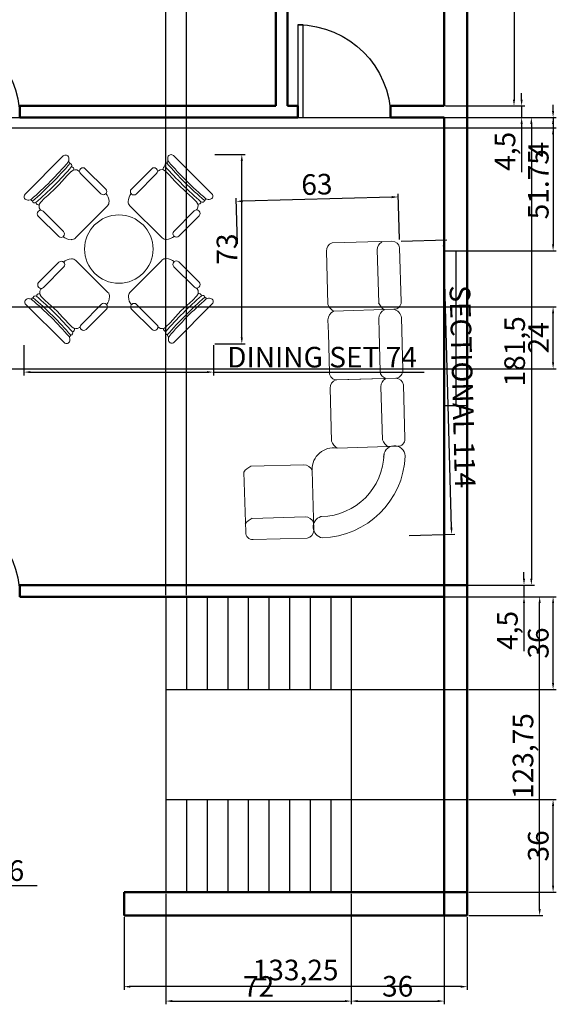
# Model space of a CAD drawing. Units: inches. Extents: x -349 to 9053, y 635 to 6001.
# Tile 4 of 7: x 540 to 749, y 636 to 1018. Entities that reach past the tile are written whole.
import ezdxf

# ---------------------------------------------------------------- set-up
doc = ezdxf.new("R2010")
doc.units = ezdxf.units.IN
for name, color, linetype, lineweight in [('A-ANNO-DIMS', 2, 'Continuous', 18), ('A-DOOR', 3, 'Continuous', 25), ('A-FLOR-STRS', 7, 'Continuous', 25), ('A-FURN', 8, 'Continuous', 18), ('A-GLAZ', 4, 'Continuous', 25), ('A-WALL', 7, 'Continuous', 50)]:
    doc.layers.add(name, color=color, linetype=linetype, lineweight=lineweight)
doc.styles.get("Standard").update_dxf_attribs({"font": 'arial.ttf'})
doc.dimstyles.new('ISO-25', dxfattribs={"dimtxt": 8, "dimasz": 2.5, "dimexe": 1.25, "dimexo": 0.625, "dimtad": 1, "dimtxsty": 'Standard', "dimcen": 2.5, "dimadec": 0, "dimazin": 0, "dimtfac": 1, "dimtmove": 0, "dimatfit": 3, "dimfxl": 1, "dimarcsym": 0})

# ---------------------------------------------------------------- blocks, each defined once
blk = doc.blocks.new('A$C054D6BE5')
at = {"ltscale": 10}
for p, q in [((-958, 560), (-569, 952)), ((559, 956), (951, 566)), ((-393, 820), (-391, 822)), ((-343, 822), (-134, 614)), ((336, 822), (128, 613)), ((386, 821), (384, 822)), ((-527, 753), (-485, 795)), ((-183, 564), (-393, 772)), ((178, 563), (386, 773)), ((478, 797), (519, 756)), ((-799, 479), (-759, 520)), ((-134, 566), (-135, 564)), ((128, 565), (130, 563)), ((752, 525), (794, 483)), ((-444, 114), (-117, 443)), ((112, 442), (442, 115)), ((-823, 387), (-825, 385)), ((-824, 337), (-615, 129)), ((-565, 179), (-775, 387)), ((563, 181), (771, 391)), ((821, 341), (613, 132)), ((819, 391), (821, 389)), ((-567, 129), (-565, 131)), ((565, 132), (563, 133)), ((-820, -342), (-612, -133)), ((-562, -182), (-770, -392)), ((-564, -133), (-562, -134)), ((-441, -116), (-111, -443)), ((441, -115), (114, -445)), ((564, -130), (562, -132)), ((562, -180), (772, -388)), ((821, -338), (612, -130)), ((-818, -392), (-819, -390)), ((820, -388), (821, -386)), ((-793, -484), (-752, -524)), ((795, -480), (755, -521)), ((-952, -566), (-559, -955)), ((-177, -564), (-385, -774)), ((-127, -566), (-129, -564)), ((130, -567), (132, -565)), ((180, -565), (390, -773)), ((955, -561), (565, -953)), ((-335, -823), (-127, -614)), ((340, -823), (131, -615)), ((-519, -756), (-477, -798)), ((524, -754), (482, -796)), ((-385, -822), (-383, -824)), ((390, -821), (388, -823))]:
    blk.add_line(p, q, dxfattribs=at)
blk.add_circle((0, 0), 350)
for centre, radius, start, end in [((-544, 928), 33.9, 14.1988, 135.2185), ((-573, 921), 63.4, 332.8301, 14.1988), ((563, 925), 63.4, 166.2382, 207.6069), ((535, 932), 33.9, 45.2185, 166.2382), ((-3237, 3211), 3575, 310.8815, 319.5555), ((-3237, 3211), 3598, 310.8815, 319.5555), ((-3237, 3211), 3632, 311.1311, 319.3059), ((-519, 874), 19.8, 10.2345, 81.0885), ((-503, 855), 22.4, 326.7437, 81.3429), ((-445, 755), 56.6, 53.5269, 135.2185), ((-488, 816), 27.1, 343.1885, 82.1651), ((-369, 796), 33.9, 135.2185, 225.2185), ((-367, 798), 33.9, 45.2185, 135.2185), ((360, 798), 33.9, 45.2185, 135.2185), ((362, 797), 33.9, 315.2185, 45.2185), ((438, 756), 56.6, 45.2185, 126.9101), ((479, 819), 27.1, 98.2719, 197.2484), ((494, 858), 22.4, 99.0941, 213.6933), ((3210, 3235), 3632, 221.1311, 229.3059), ((510, 877), 19.8, 99.3484, 170.2025), ((3210, 3235), 3598, 220.8815, 229.5555), ((3210, 3235), 3575, 220.8815, 229.5555), ((-2165, 2147), 2151, 310.8397, 319.5973), ((-2445, -1950), 3420, 53.3465, 53.5269), ((2458, -1933), 3420, 126.9101, 127.0905), ((2146, 2163), 2151, 220.8397, 229.5973), ((-158, 590), 33.9, 315.2185, 45.2185), ((152, 589), 33.9, 135.2185, 225.2185), ((-934, 536), 33.9, 135.2185, 256.2382), ((-927, 564), 63.4, 256.2382, 297.6069), ((-879, 511), 19.8, 189.3484, 260.2025), ((-159, 588), 33.9, 225.2185, 315.2185), ((-247, 477), 147, 4.1611, 38.3267), ((242, 477), 147, 142.1103, 176.2759), ((154, 587), 33.9, 225.2185, 315.2185), ((873, 517), 19.8, 280.2345, 351.0885), ((920, 571), 63.4, 242.8301, 284.1988), ((927, 542), 33.9, 284.1988, 45.2185), ((-861, 495), 22.4, 189.0941, 303.6933), ((-821, 480), 27.1, 188.2719, 287.2484), ((-759, 439), 56.6, 135.2185, 216.9101), ((1931, 2460), 3420, 216.9101, 217.0905), ((-157, 483), 56.6, 315.2185, 4.1611), ((152, 482), 56.6, 176.2759, 225.2185), ((-1951, 2443), 3420, 323.3465, 323.5269), ((754, 443), 56.6, 323.5269, 45.2185), ((815, 486), 27.1, 253.1885, 352.1651), ((854, 501), 22.4, 236.7437, 351.3429), ((-800, 361), 33.9, 135.2185, 225.2185), ((-799, 363), 33.9, 45.2185, 135.2185), ((795, 367), 33.9, 45.2185, 135.2185), ((797, 365), 33.9, 315.2185, 45.2185), ((-591, 153), 33.9, 225.2185, 315.2185), ((-479, 243), 147, 232.1103, 266.2759), ((-589, 155), 33.9, 315.2185, 45.2185), ((-484, 153), 56.6, 266.2759, 315.2185), ((482, 155), 56.6, 225.2185, 274.1611), ((476, 245), 147, 274.1611, 308.3267), ((587, 157), 33.9, 135.2185, 225.2185), ((589, 156), 33.9, 225.2185, 315.2185), ((-475, -246), 147, 94.1611, 128.3267), ((-481, -156), 56.6, 45.2185, 94.1611), ((481, -154), 56.6, 86.2759, 135.2185), ((475, -244), 147, 52.1103, 86.2759), ((-588, -157), 33.9, 45.2185, 135.2185), ((-586, -158), 33.9, 315.2185, 45.2185), ((586, -156), 33.9, 135.2185, 225.2185), ((588, -154), 33.9, 45.2185, 135.2185), ((-796, -366), 33.9, 135.2185, 225.2185), ((-794, -368), 33.9, 225.2185, 315.2185), ((1952, -2444), 3420, 143.3465, 143.5269), ((796, -364), 33.9, 225.2185, 315.2185), ((-1934, -2461), 3420, 36.9101, 37.0905), ((797, -362), 33.9, 315.2185, 45.2185), ((-873, -516), 19.8, 100.2345, 171.0885), ((-855, -500), 22.4, 56.7437, 171.3429), ((-3211, -3235), 3598, 40.8815, 49.5555), ((-3211, -3235), 3632, 41.1311, 49.3059), ((-816, -485), 27.1, 73.1885, 172.1651), ((-753, -444), 56.6, 143.5269, 225.2185), ((-241, -478), 147, 322.1103, 356.2759), ((-151, -483), 56.6, 356.2759, 45.2185), ((154, -484), 56.6, 135.2185, 184.1611), ((244, -478), 147, 184.1611, 218.3267), ((3234, -3212), 3632, 131.1311, 139.3059), ((3234, -3212), 3598, 130.8815, 139.5555), ((755, -440), 56.6, 315.2185, 36.9101), ((818, -481), 27.1, 8.2719, 107.2484), ((857, -496), 22.4, 9.0941, 123.6933), ((876, -512), 19.8, 9.3484, 80.2025), ((924, -565), 63.4, 76.2382, 117.6069), ((-928, -542), 33.9, 104.1988, 225.2185), ((-920, -570), 63.4, 62.8301, 104.1988), ((-3211, -3235), 3575, 40.8815, 49.5555), ((-2147, -2163), 2151, 40.8397, 49.5973), ((-153, -588), 33.9, 45.2185, 135.2185), ((-151, -590), 33.9, 315.2185, 45.2185), ((155, -591), 33.9, 135.2185, 225.2185), ((156, -589), 33.9, 45.2185, 135.2185), ((3234, -3212), 3575, 130.8815, 139.5555), ((2162, -2148), 2151, 130.8397, 139.5973), ((931, -537), 33.9, 315.2185, 76.2382), ((-437, -757), 56.6, 225.2185, 306.9101), ((-2457, 1932), 3420, 306.9101, 307.0905), ((-361, -798), 33.9, 135.2185, 225.2185), ((366, -797), 33.9, 315.2185, 45.2185), ((2442, 1949), 3420, 233.3465, 233.5269), ((442, -756), 56.6, 233.5269, 315.2185), ((-564, -924), 63.4, 346.2382, 27.6069), ((-510, -877), 19.8, 279.3484, 350.2025), ((-494, -858), 22.4, 279.0941, 33.6933), ((-479, -819), 27.1, 278.2719, 17.2484), ((-359, -799), 33.9, 225.2185, 315.2185), ((364, -799), 33.9, 225.2185, 315.2185), ((485, -817), 27.1, 163.1885, 262.1651), ((500, -856), 22.4, 146.7437, 261.3429), ((516, -875), 19.8, 190.2345, 261.0885), ((570, -922), 63.4, 152.8301, 194.1988), ((-535, -931), 33.9, 225.2185, 346.2382), ((541, -929), 33.9, 194.1988, 315.2185)]:
    blk.add_arc(centre, radius, start, end, dxfattribs=at)
blk = doc.blocks.new('A$C5F6A1817')
for p, q in [((0.807, 1.928, -342.856), (0.09, 1.925, -342.856)), ((0.001, 1.196, -342.856), (0.001, 1.84, -342.856)), ((0.254, 1.843, -342.856), (0.254, 1.211, -342.856)), ((0.874, 1.843, -342.856), (0.874, 1.211, -342.856)), ((0.804, 1.115, -342.856), (0.09, 1.115, -342.856)), ((0.183, 1.115, -342.856), (0.181, 1.115, -342.856)), ((0.252, 1.026, -342.856), (0.252, 1.017, -342.856)), ((1.146, 0.873, -342.856), (1.779, 0.873, -342.856)), ((1.96, 0.876, -342.856), (2.433, 0.876, -342.856)), ((2.433, 0.876, -342.856), (2.592, 0.876, -342.856)), ((2.777, 0.873, -342.856), (3.41, 0.873, -342.856)), ((1.064, 0.089, -342.856), (1.061, 0.806, -342.856)), ((1.875, 0.802, -342.856), (1.875, 0.089, -342.856)), ((1.875, 0.081, -342.856), (1.875, 0.791, -342.856)), ((2.696, 0.089, -342.856), (2.692, 0.806, -342.856)), ((3.506, 0.802, -342.856), (3.506, 0.089, -342.856)), ((1.146, 0.267, -342.856), (1.779, 0.267, -342.856)), ((1.96, 0.271, -342.856), (2.433, 0.271, -342.856)), ((2.433, 0.271, -342.856), (2.592, 0.271, -342.856)), ((2.777, 0.267, -342.856), (3.41, 0.267, -342.856)), ((1.793, 0, -342.856), (1.15, 0, -342.856)), ((2.596, 0, -342.856), (1.971, 0, -342.856)), ((3.425, 0, -342.856), (2.781, 0, -342.856))]:
    blk.add_line(p, q)
for centre, radius, start, end in [((0.086, 1.84, -342.856), 0.0852, 87.5912, 180), ((0.063, 1.762, -342.856), 0.208, 22.9498, 53.1162), ((0.683, 1.762, -342.856), 0.208, 22.9498, 53.1162), ((0.09, 1.204, -342.856), 0.0891, 184.9502, 270), ((0.153, 1.211, -342.856), 0.101, 287.7112, 0), ((0.773, 1.211, -342.856), 0.101, 287.7112, 0), ((0.127, 0.988, -342.856), 0.131, 16.7665, 167.5739), ((0.813, 0.858, -342.856), 0.255, 349.3994, 90), ((1.018, 1.017, -342.856), 1.018, 180.0517, 266.013), ((1.018, 1.017, -342.856), 0.766, 180, 267.0841), ((1.227, 0.682, -342.856), 0.208, 112.9498, 143.1162), ((1.779, 0.772, -342.856), 0.101, 17.7112, 90), ((1.96, 0.791, -342.856), 0.085, 89.971, 180), ((2.592, 0.77, -342.856), 0.106, 19.7589, 90), ((2.858, 0.682, -342.856), 0.208, 112.9498, 143.1162), ((3.41, 0.772, -342.856), 0.101, 17.7112, 90), ((0.942, 0.13, -342.856), 0.129, 271.9879, 91.9879), ((1.227, 0.076, -342.856), 0.208, 112.9498, 143.1162), ((1.779, 0.166, -342.856), 0.101, 25.9257, 90), ((1.96, 0.186, -342.856), 0.085, 89.971, 163.2423), ((2.592, 0.164, -342.856), 0.106, 19.7589, 90), ((2.858, 0.076, -342.856), 0.208, 112.9498, 143.1162), ((3.41, 0.166, -342.856), 0.101, 25.9257, 90), ((1.15, 0.085, -342.856), 0.0852, 177.5912, 270), ((1.786, 0.089, -342.856), 0.0891, 274.9502, 0), ((1.971, 0.098, -342.856), 0.0975, 189.5558, 270), ((2.575, 0.124, -342.856), 0.126, 279.5063, 343.732), ((2.781, 0.085, -342.856), 0.0852, 177.5912, 270), ((3.417, 0.089, -342.856), 0.0891, 274.9502, 0)]:
    blk.add_arc(centre, radius, start, end)
blk = doc.blocks.new('*D30')
at = {"layer": 'A-ANNO-DIMS', "color": 0, "lineweight": -2, "transparency": 16777216}
for p, q in [((580.75, 669.38), (580.75, 641.1)), ((714, 669.38), (714, 641.1)), ((711.5, 642.35), (583.25, 642.35))]:
    blk.add_line(p, q, dxfattribs=at)
at = {"layer": 'A-ANNO-DIMS', "color": 0, "transparency": 16777216}
for points in [[(583.25, 642.77), (583.25, 641.93), (580.75, 642.35)], [(711.5, 642.77), (711.5, 641.93), (714, 642.35)]]:
    blk.add_solid(points, dxfattribs=at)
at = {"layer": 'Defpoints', "color": 0, "transparency": 16777216}
for p in [(580.75, 670), (714, 670), (580.75, 642.35)]:
    blk.add_point(p, dxfattribs=at)
at = {"layer": 'A-ANNO-DIMS', "color": 0, "transparency": 16777216, "insert": (647.37, 647.78), "char_height": 8, "attachment_point": 5}
blk.add_mtext('133,25', dxfattribs=at)
blk = doc.blocks.new('*D32')
at = {"layer": 'A-ANNO-DIMS', "color": 0, "lineweight": -2, "transparency": 16777216}
for p, q in [((705.63, 1117), (733.43, 1117)), ((732.18, 1114.5), (732.18, 986.75)), ((705.63, 984.25), (733.43, 984.25))]:
    blk.add_line(p, q, dxfattribs=at)
at = {"layer": 'A-ANNO-DIMS', "color": 0, "transparency": 16777216}
for points in [[(731.76, 1114.5), (732.59, 1114.5), (732.18, 1117)], [(731.76, 986.75), (732.59, 986.75), (732.18, 984.25)]]:
    blk.add_solid(points, dxfattribs=at)
at = {"layer": 'Defpoints', "color": 0, "transparency": 16777216}
for p in [(705, 1117), (705, 984.25), (732.18, 984.25)]:
    blk.add_point(p, dxfattribs=at)
at = {"layer": 'A-ANNO-DIMS', "color": 0, "transparency": 16777216, "insert": (726.74, 1050.62), "char_height": 8, "attachment_point": 5, "rotation": 90}
blk.add_mtext('132,75', dxfattribs=at)
blk = doc.blocks.new('*D33')
at = {"layer": 'A-ANNO-DIMS', "color": 0, "lineweight": -2, "transparency": 16777216}
for p, q in [((735.13, 986.75), (735.13, 989.25)), ((705.63, 984.25), (736.38, 984.25)), ((735.13, 984.25), (735.13, 979.75)), ((705.63, 979.75), (736.38, 979.75)), ((735.13, 977.25), (735.13, 958.55))]:
    blk.add_line(p, q, dxfattribs=at)
at = {"layer": 'A-ANNO-DIMS', "color": 0, "transparency": 16777216}
for points in [[(734.71, 986.75), (735.55, 986.75), (735.13, 984.25)], [(734.71, 977.25), (735.55, 977.25), (735.13, 979.75)]]:
    blk.add_solid(points, dxfattribs=at)
at = {"layer": 'Defpoints', "color": 0, "transparency": 16777216}
for p in [(705, 984.25), (705, 979.75), (735.13, 979.75)]:
    blk.add_point(p, dxfattribs=at)
at = {"layer": 'A-ANNO-DIMS', "color": 0, "transparency": 16777216, "insert": (729.71, 966.65), "char_height": 8, "attachment_point": 5, "rotation": 90}
blk.add_mtext('4,5', dxfattribs=at)
blk = doc.blocks.new('*D34')
at = {"layer": 'A-ANNO-DIMS', "color": 0, "lineweight": -2, "transparency": 16777216}
for p, q in [((705.63, 979.75), (740.16, 979.75)), ((738.91, 977.25), (738.91, 800.75)), ((705.63, 798.25), (740.16, 798.25))]:
    blk.add_line(p, q, dxfattribs=at)
at = {"layer": 'A-ANNO-DIMS', "color": 0, "transparency": 16777216}
for points in [[(738.49, 977.25), (739.32, 977.25), (738.91, 979.75)], [(738.49, 800.75), (739.32, 800.75), (738.91, 798.25)]]:
    blk.add_solid(points, dxfattribs=at)
at = {"layer": 'Defpoints', "color": 0, "transparency": 16777216}
for p in [(705, 979.75), (705, 798.25), (738.91, 798.25)]:
    blk.add_point(p, dxfattribs=at)
at = {"layer": 'A-ANNO-DIMS', "color": 0, "transparency": 16777216, "insert": (733.47, 889), "char_height": 8, "attachment_point": 5, "rotation": 90}
blk.add_mtext('181,5', dxfattribs=at)
blk = doc.blocks.new('*D35')
at = {"layer": 'A-ANNO-DIMS', "color": 0, "lineweight": -2, "transparency": 16777216}
for p, q in [((736.05, 800.75), (736.05, 803.25)), ((705.63, 798.25), (737.3, 798.25)), ((736.05, 798.25), (736.05, 793.75)), ((705.63, 793.75), (737.3, 793.75)), ((736.05, 791.25), (736.05, 772.55))]:
    blk.add_line(p, q, dxfattribs=at)
at = {"layer": 'A-ANNO-DIMS', "color": 0, "transparency": 16777216}
for points in [[(735.64, 800.75), (736.47, 800.75), (736.05, 798.25)], [(735.64, 791.25), (736.47, 791.25), (736.05, 793.75)]]:
    blk.add_solid(points, dxfattribs=at)
at = {"layer": 'Defpoints', "color": 0, "transparency": 16777216}
for p in [(705, 798.25), (705, 793.75), (736.05, 793.75)]:
    blk.add_point(p, dxfattribs=at)
at = {"layer": 'A-ANNO-DIMS', "color": 0, "transparency": 16777216, "insert": (730.64, 780.65), "char_height": 8, "attachment_point": 5, "rotation": 90}
blk.add_mtext('4,5', dxfattribs=at)
blk = doc.blocks.new('*D36')
at = {"layer": 'A-ANNO-DIMS', "color": 0, "lineweight": -2, "transparency": 16777216}
for p, q in [((714.63, 793.75), (743.38, 793.75)), ((742.13, 672.5), (742.13, 791.25)), ((714.63, 670), (743.38, 670))]:
    blk.add_line(p, q, dxfattribs=at)
at = {"layer": 'A-ANNO-DIMS', "color": 0, "transparency": 16777216}
for points in [[(741.71, 791.25), (742.55, 791.25), (742.13, 793.75)], [(741.71, 672.5), (742.55, 672.5), (742.13, 670)]]:
    blk.add_solid(points, dxfattribs=at)
at = {"layer": 'Defpoints', "color": 0, "transparency": 16777216}
for p in [(714, 793.75), (742.13, 793.75), (714, 670)]:
    blk.add_point(p, dxfattribs=at)
at = {"layer": 'A-ANNO-DIMS', "color": 0, "transparency": 16777216, "insert": (736.7, 731.88), "char_height": 8, "attachment_point": 5, "rotation": 90}
blk.add_mtext('123,75', dxfattribs=at)
blk = doc.blocks.new('DOOR-36IN-SWING')
blk.add_line((0, 0), (-2, 0))
blk.add_lwpolyline([(0, 36), (0, 0), (-2, 0), (-2, 36)], close=True)
blk.add_arc((0, 0), 36, 90, 180)
blk = doc.blocks.new('WIN-60IN')
for p, q in [((0, -4.5), (0, 4.5)), ((60, -4.5), (60, 4.5)), ((0, 0), (60, 0))]:
    blk.add_line(p, q)
blk = doc.blocks.new('*D41')
at = {"layer": 'A-ANNO-DIMS', "color": 0, "lineweight": -2, "transparency": 16777216}
for p, q in [((387, 686.37), (387, 680.35)), ((423, 686.37), (423, 680.35)), ((389.5, 681.6), (420.5, 681.6)), ((423, 681.6), (547.07, 681.6))]:
    blk.add_line(p, q, dxfattribs=at)
at = {"layer": 'A-ANNO-DIMS', "color": 0, "transparency": 16777216}
for points in [[(389.5, 682.02), (389.5, 681.18), (387, 681.6)], [(420.5, 682.02), (420.5, 681.18), (423, 681.6)]]:
    blk.add_solid(points, dxfattribs=at)
at = {"layer": 'Defpoints', "color": 0, "transparency": 16777216}
for p in [(387, 687), (423, 687), (423, 681.6)]:
    blk.add_point(p, dxfattribs=at)
at = {"layer": 'A-ANNO-DIMS', "color": 0, "transparency": 16777216, "insert": (486.29, 686.37), "char_height": 8, "attachment_point": 5}
blk.add_mtext('THRESHOLD DOOR 36', dxfattribs=at)
blk = doc.blocks.new('*D55')
at = {"layer": 'A-ANNO-DIMS', "color": 0, "lineweight": -2, "transparency": 16777216}
for p, q in [((541.92, 891.34), (541.92, 879.68)), ((615.46, 891.34), (615.46, 879.68)), ((544.42, 880.93), (612.96, 880.93)), ((615.46, 880.93), (697.3, 880.93))]:
    blk.add_line(p, q, dxfattribs=at)
at = {"layer": 'A-ANNO-DIMS', "color": 0, "transparency": 16777216}
for points in [[(544.42, 881.35), (544.42, 880.51), (541.92, 880.93)], [(612.96, 881.35), (612.96, 880.51), (615.46, 880.93)]]:
    blk.add_solid(points, dxfattribs=at)
at = {"layer": 'Defpoints', "color": 0, "transparency": 16777216}
for p in [(541.92, 891.96), (615.46, 891.96), (615.46, 880.93)]:
    blk.add_point(p, dxfattribs=at)
at = {"layer": 'A-ANNO-DIMS', "color": 0, "transparency": 16777216, "insert": (657.63, 885.69), "char_height": 8, "attachment_point": 5}
blk.add_mtext('DINING SET 74', dxfattribs=at)
blk = doc.blocks.new('*D56')
at = {"layer": 'A-ANNO-DIMS', "color": 0, "lineweight": -2, "transparency": 16777216}
for p, q in [((616.08, 965.44), (627.74, 965.44)), ((626.49, 894.46), (626.49, 962.94)), ((616.08, 891.96), (627.74, 891.96))]:
    blk.add_line(p, q, dxfattribs=at)
at = {"layer": 'A-ANNO-DIMS', "color": 0, "transparency": 16777216}
for points in [[(626.07, 962.94), (626.9, 962.94), (626.49, 965.44)], [(626.07, 894.46), (626.9, 894.46), (626.49, 891.96)]]:
    blk.add_solid(points, dxfattribs=at)
at = {"layer": 'Defpoints', "color": 0, "transparency": 16777216}
for p in [(615.46, 965.44), (626.49, 965.44), (615.46, 891.96)]:
    blk.add_point(p, dxfattribs=at)
at = {"layer": 'A-ANNO-DIMS', "color": 0, "transparency": 16777216, "insert": (621.77, 928.7), "char_height": 8, "attachment_point": 5, "rotation": 90}
blk.add_mtext('73', dxfattribs=at)
blk = doc.blocks.new('*D57')
at = {"layer": 'A-ANNO-DIMS', "color": 0, "lineweight": -2, "transparency": 16777216}
for p, q in [((688.31, 931.82), (706.08, 932.3)), ((707.89, 820.49), (704.89, 929.77)), ((691.44, 817.54), (709.21, 818.03))]:
    blk.add_line(p, q, dxfattribs=at)
at = {"layer": 'A-ANNO-DIMS', "color": 0, "transparency": 16777216}
for points in [[(705.31, 929.78), (704.48, 929.76), (704.83, 932.27)], [(708.31, 820.5), (707.47, 820.48), (707.96, 817.99)]]:
    blk.add_solid(points, dxfattribs=at)
at = {"layer": 'Defpoints', "color": 0, "transparency": 16777216}
for p in [(687.68, 931.8), (704.83, 932.27), (690.82, 817.52)]:
    blk.add_point(p, dxfattribs=at)
at = {"layer": 'A-ANNO-DIMS', "color": 0, "transparency": 16777216, "insert": (711.16, 875.26), "char_height": 8, "attachment_point": 5, "rotation": 271.571}
blk.add_mtext('SECTIONAL 114', dxfattribs=at)
blk = doc.blocks.new('*D58')
at = {"layer": 'A-ANNO-DIMS', "color": 0, "lineweight": -2, "transparency": 16777216}
for p, q in [((624.81, 930.7), (624.33, 948.47)), ((684.72, 948.87), (626.86, 947.29)), ((687.67, 932.42), (687.18, 950.19))]:
    blk.add_line(p, q, dxfattribs=at)
at = {"layer": 'A-ANNO-DIMS', "color": 0, "transparency": 16777216}
for points in [[(684.7, 949.29), (684.73, 948.46), (687.21, 948.94)], [(626.85, 947.7), (626.87, 946.87), (624.36, 947.22)]]:
    blk.add_solid(points, dxfattribs=at)
at = {"layer": 'Defpoints', "color": 0, "transparency": 16777216}
for p in [(624.36, 947.22), (624.83, 930.08), (687.68, 931.8)]:
    blk.add_point(p, dxfattribs=at)
at = {"layer": 'A-ANNO-DIMS', "color": 0, "transparency": 16777216, "insert": (655.66, 952.79), "char_height": 8, "attachment_point": 5, "rotation": 1.571}
blk.add_mtext('63', dxfattribs=at)
blk = doc.blocks.new('*D61')
at = {"layer": 'A-ANNO-DIMS', "color": 0, "lineweight": -2, "transparency": 16777216}
for p, q in [((435.63, 906.25), (748.6, 906.25)), ((747.35, 884.75), (747.35, 903.75)), ((435.63, 882.25), (748.6, 882.25))]:
    blk.add_line(p, q, dxfattribs=at)
at = {"layer": 'A-ANNO-DIMS', "color": 0, "transparency": 16777216}
for points in [[(746.93, 903.75), (747.76, 903.75), (747.35, 906.25)], [(746.93, 884.75), (747.76, 884.75), (747.35, 882.25)]]:
    blk.add_solid(points, dxfattribs=at)
at = {"layer": 'Defpoints', "color": 0, "transparency": 16777216}
for p in [(435, 906.25), (747.35, 906.25), (435, 882.25)]:
    blk.add_point(p, dxfattribs=at)
at = {"layer": 'A-ANNO-DIMS', "color": 0, "transparency": 16777216, "insert": (742.71, 894.25), "char_height": 8, "attachment_point": 5, "rotation": 90}
blk.add_mtext('24', dxfattribs=at)
blk = doc.blocks.new('*D63')
at = {"layer": 'A-ANNO-DIMS', "color": 0, "lineweight": -2, "transparency": 16777216}
for p, q in [((747.35, 982.25), (747.35, 984.75)), ((440.13, 979.75), (748.6, 979.75)), ((747.35, 979.75), (747.35, 975.75)), ((440.13, 975.75), (748.6, 975.75)), ((747.35, 973.25), (747.35, 963.97))]:
    blk.add_line(p, q, dxfattribs=at)
at = {"layer": 'A-ANNO-DIMS', "color": 0, "transparency": 16777216}
for points in [[(746.93, 982.25), (747.76, 982.25), (747.35, 979.75)], [(746.93, 973.25), (747.76, 973.25), (747.35, 975.75)]]:
    blk.add_solid(points, dxfattribs=at)
at = {"layer": 'Defpoints', "color": 0, "transparency": 16777216}
for p in [(439.5, 979.75), (439.5, 975.75), (747.35, 975.75)]:
    blk.add_point(p, dxfattribs=at)
at = {"layer": 'A-ANNO-DIMS', "color": 0, "transparency": 16777216, "insert": (742.72, 967.36), "char_height": 8, "attachment_point": 5, "rotation": 90}
blk.add_mtext('4', dxfattribs=at)
blk = doc.blocks.new('*D64')
at = {"layer": 'A-ANNO-DIMS', "color": 0, "lineweight": -2, "transparency": 16777216}
for p, q in [((597, 678.38), (597, 635.5)), ((669, 678.38), (669, 635.5)), ((599.5, 636.75), (666.5, 636.75))]:
    blk.add_line(p, q, dxfattribs=at)
at = {"layer": 'A-ANNO-DIMS', "color": 0, "transparency": 16777216}
for points in [[(599.5, 637.17), (599.5, 636.33), (597, 636.75)], [(666.5, 637.17), (666.5, 636.33), (669, 636.75)]]:
    blk.add_solid(points, dxfattribs=at)
at = {"layer": 'Defpoints', "color": 0, "transparency": 16777216}
for p in [(597, 679), (669, 679), (669, 636.75)]:
    blk.add_point(p, dxfattribs=at)
at = {"layer": 'A-ANNO-DIMS', "color": 0, "transparency": 16777216, "insert": (633, 641.39), "char_height": 8, "attachment_point": 5}
blk.add_mtext('72', dxfattribs=at)
blk = doc.blocks.new('*D65')
at = {"layer": 'A-ANNO-DIMS', "color": 0, "lineweight": -2, "transparency": 16777216}
for p, q in [((669, 678.38), (669, 635.5)), ((705, 678.38), (705, 635.5)), ((671.5, 636.75), (702.5, 636.75))]:
    blk.add_line(p, q, dxfattribs=at)
at = {"layer": 'A-ANNO-DIMS', "color": 0, "transparency": 16777216}
for points in [[(671.5, 637.17), (671.5, 636.33), (669, 636.75)], [(702.5, 637.17), (702.5, 636.33), (705, 636.75)]]:
    blk.add_solid(points, dxfattribs=at)
at = {"layer": 'Defpoints', "color": 0, "transparency": 16777216}
for p in [(669, 679), (705, 679), (705, 636.75)]:
    blk.add_point(p, dxfattribs=at)
at = {"layer": 'A-ANNO-DIMS', "color": 0, "transparency": 16777216, "insert": (687, 641.46), "char_height": 8, "attachment_point": 5}
blk.add_mtext('36', dxfattribs=at)
blk = doc.blocks.new('*D66')
at = {"layer": 'A-ANNO-DIMS', "color": 0, "lineweight": -2, "transparency": 16777216}
for p, q in [((714.63, 715), (748.6, 715)), ((747.35, 681.5), (747.35, 712.5)), ((714.63, 679), (748.6, 679))]:
    blk.add_line(p, q, dxfattribs=at)
at = {"layer": 'A-ANNO-DIMS', "color": 0, "transparency": 16777216}
for points in [[(746.93, 712.5), (747.76, 712.5), (747.35, 715)], [(746.93, 681.5), (747.76, 681.5), (747.35, 679)]]:
    blk.add_solid(points, dxfattribs=at)
at = {"layer": 'Defpoints', "color": 0, "transparency": 16777216}
for p in [(714, 715), (747.35, 715), (714, 679)]:
    blk.add_point(p, dxfattribs=at)
at = {"layer": 'A-ANNO-DIMS', "color": 0, "transparency": 16777216, "insert": (742.63, 697), "char_height": 8, "attachment_point": 5, "rotation": 90}
blk.add_mtext('36', dxfattribs=at)
blk = doc.blocks.new('*D67')
at = {"layer": 'A-ANNO-DIMS', "color": 0, "lineweight": -2, "transparency": 16777216}
for p, q in [((705.63, 793.75), (748.6, 793.75)), ((747.35, 760.25), (747.35, 791.25)), ((714.63, 757.75), (748.6, 757.75))]:
    blk.add_line(p, q, dxfattribs=at)
at = {"layer": 'A-ANNO-DIMS', "color": 0, "transparency": 16777216}
for points in [[(746.93, 791.25), (747.76, 791.25), (747.35, 793.75)], [(746.93, 760.25), (747.76, 760.25), (747.35, 757.75)]]:
    blk.add_solid(points, dxfattribs=at)
at = {"layer": 'Defpoints', "color": 0, "transparency": 16777216}
for p in [(705, 793.75), (747.35, 793.75), (714, 757.75)]:
    blk.add_point(p, dxfattribs=at)
at = {"layer": 'A-ANNO-DIMS', "color": 0, "transparency": 16777216, "insert": (742.63, 775.75), "char_height": 8, "attachment_point": 5, "rotation": 90}
blk.add_mtext('36', dxfattribs=at)
blk = doc.blocks.new('*D68')
at = {"layer": 'A-ANNO-DIMS', "color": 0, "lineweight": -2, "transparency": 16777216}
for p, q in [((597, 794.38), (597, 1160.5)), ((599.5, 1159.25), (602.5, 1159.25)), ((605, 794.38), (605, 1160.5))]:
    blk.add_line(p, q, dxfattribs=at)
at = {"layer": 'A-ANNO-DIMS', "color": 0, "transparency": 16777216}
for points in [[(599.5, 1159.67), (599.5, 1158.83), (597, 1159.25)], [(602.5, 1159.67), (602.5, 1158.83), (605, 1159.25)]]:
    blk.add_solid(points, dxfattribs=at)
at = {"layer": 'Defpoints', "color": 0, "transparency": 16777216}
for p in [(605, 1159.25), (597, 793.75), (605, 793.75)]:
    blk.add_point(p, dxfattribs=at)
at = {"layer": 'A-ANNO-DIMS', "color": 0, "transparency": 16777216, "insert": (601, 1163.96), "char_height": 8, "attachment_point": 5}
blk.add_mtext('8', dxfattribs=at)
blk = doc.blocks.new('*D73')
at = {"layer": 'A-ANNO-DIMS', "color": 0, "lineweight": -2, "transparency": 16777216}
for p, q in [((705.63, 979.75), (748.6, 979.75)), ((747.35, 977.25), (747.35, 930.5)), ((705.72, 928), (748.6, 928))]:
    blk.add_line(p, q, dxfattribs=at)
at = {"layer": 'A-ANNO-DIMS', "color": 0, "transparency": 16777216}
for points in [[(746.93, 977.25), (747.76, 977.25), (747.35, 979.75)], [(746.93, 930.5), (747.76, 930.5), (747.35, 928)]]:
    blk.add_solid(points, dxfattribs=at)
at = {"layer": 'Defpoints', "color": 0, "transparency": 16777216}
for p in [(705, 979.75), (705.1, 928), (747.35, 928)]:
    blk.add_point(p, dxfattribs=at)
at = {"layer": 'A-ANNO-DIMS', "color": 0, "transparency": 16777216, "insert": (742.64, 953.88), "char_height": 8, "attachment_point": 5, "rotation": 90}
blk.add_mtext('51.75', dxfattribs=at)

msp = doc.modelspace()

# ---------------------------------------------------------------- linework, layer by layer
at = {"layer": 'A-FLOR-STRS'}
for p, q in [((597, 793.75), (597, 679)), ((605, 793.75), (605, 757.75)), ((605, 793.75), (605, 757.75)), ((613, 793.75), (613, 757.75)), ((613, 793.75), (613, 757.75)), ((621, 793.75), (621, 757.75)), ((621, 793.75), (621, 757.75)), ((629, 793.75), (629, 757.75)), ((629, 793.75), (629, 757.75)), ((637, 793.75), (637, 757.75)), ((637, 793.75), (637, 757.75)), ((645, 793.75), (645, 757.75)), ((645, 793.75), (645, 757.75)), ((653, 793.75), (653, 757.75)), ((653, 793.75), (653, 757.75)), ((661, 793.75), (661, 757.75)), ((661, 793.75), (661, 757.75)), ((669, 793.75), (669, 679)), ((705, 793.75), (705, 679)), ((597, 757.75), (714, 757.75)), ((597, 715), (714, 715)), ((605, 715), (605, 679)), ((605, 715), (605, 679)), ((613, 715), (613, 679)), ((613, 715), (613, 679)), ((621, 715), (621, 679)), ((621, 715), (621, 679)), ((629, 715), (629, 679)), ((629, 715), (629, 679)), ((637, 715), (637, 679)), ((637, 715), (637, 679)), ((645, 715), (645, 679)), ((645, 715), (645, 679)), ((653, 715), (653, 679)), ((653, 715), (653, 679)), ((661, 715), (661, 679)), ((661, 715), (661, 679))]:
    msp.add_line(p, q, dxfattribs=at)
at = {"layer": 'A-WALL'}
for p, q in [((714, 670), (714, 1126)), ((639.75, 1117), (639.75, 984.25)), ((644.25, 1117), (644.25, 984.25)), ((705, 984.25), (705, 1117)), ((540.25, 984.25), (540.25, 979.75)), ((540.25, 984.25), (639.75, 984.25)), ((644.25, 984.25), (648.25, 984.25)), ((648.25, 984.25), (648.25, 979.75)), ((684.25, 984.25), (684.25, 979.75)), ((684.25, 984.25), (705, 984.25)), ((540.25, 979.75), (648.25, 979.75)), ((684.25, 979.75), (705, 979.75)), ((705, 670), (705, 979.75)), ((705, 798.25), (705, 979.75)), ((705, 979.75), (705, 798.25)), ((540.25, 793.75), (540.25, 798.25)), ((540.25, 798.25), (714, 798.25)), ((540.25, 793.75), (705, 793.75)), ((580.75, 679), (580.75, 670)), ((580.75, 679), (714, 679)), ((580.75, 670), (714, 670))]:
    msp.add_line(p, q, dxfattribs=at)

# ---------------------------------------------------------------- block references
at = {"layer": 'A-DOOR', "extrusion": (0, 0, -1), "zscale": -1}
for p in [(-504.25, 979.75), (-648.25, 979.75), (-504.25, 793.75)]:
    msp.add_blockref('DOOR-36IN-SWING', p, dxfattribs=at)
at = {"layer": 'A-FURN', "xscale": 0.0379749276700036, "yscale": 0.0379749276700036, "zscale": 0.0379749276700036}
msp.add_blockref('A$C054D6BE5', (578.7457, 928.6905), dxfattribs=at)
at = {"layer": 'A-FURN', "xscale": 32.60612297228437, "yscale": 32.60612297228437, "zscale": 32.60612297228437, "rotation": 91.57097422574253}
msp.add_blockref('A$C5F6A1817', (690.8184, 817.5231, 11179.209), dxfattribs=at)
at = {"layer": 'A-GLAZ', "rotation": 270}
msp.add_blockref('WIN-60IN', (709.5971, 928), dxfattribs=at)

# ---------------------------------------------------------------- dimensions: what is measured, and where the dimension line sits
at = {"layer": 'A-ANNO-DIMS'}
for base, p1, p2, override, picture, middle in [((605, 1159.25), (597, 793.75), (605, 793.75), {"dimdec": 0, "dimlfac": 1, "dimrnd": 0, "dimzin": 0, "dimdsep": 46, "dimlunit": 2}, '*D68', (601, 1163.9596)), ((669, 636.75), (597, 679), (669, 679), {"dimdec": 0, "dimlfac": 1, "dimrnd": 0, "dimzin": 0, "dimdsep": 46, "dimlunit": 2}, '*D64', (633, 641.3914)), ((705, 636.75), (669, 679), (705, 679), {"dimdec": 0, "dimlfac": 1, "dimrnd": 0, "dimzin": 0, "dimdsep": 46, "dimlunit": 2}, '*D65', (687, 641.4623)), ((580.75, 642.3504), (714, 670), (580.75, 670), {"dimclrd": 0, "dimclre": 0, "dimclrt": 0}, '*D30', (647.375, 647.7831))]:
    dim = msp.add_linear_dim(base=base, p1=p1, p2=p2, dimstyle='ISO-25', override=override, dxfattribs=at)
    dim.commit()
    dim.dimension.update_dxf_attribs({"geometry": picture, "text_midpoint": middle})
for base, p1, p2, angle, override, picture, middle in [((732.1753, 984.25), (705, 1117), (705, 984.25), 90, {"dimclrd": 0, "dimclre": 0, "dimclrt": 0}, '*D32', (726.7426, 1050.625)), ((735.1289, 979.75), (705, 984.25), (705, 979.75), 90, {"dimclrd": 0, "dimclre": 0, "dimclrt": 0}, '*D33', (729.7126, 966.6516)), ((747.3471, 975.75), (439.5, 979.75), (439.5, 975.75), 90, {"dimdec": 0, "dimlfac": 1, "dimrnd": 0, "dimzin": 0, "dimdsep": 46, "dimlunit": 2}, '*D63', (742.7221, 967.3583)), ((738.9056, 798.25), (705, 979.75), (705, 798.25), 90, {"dimclrd": 0, "dimclre": 0, "dimclrt": 0}, '*D34', (733.473, 889)), ((747.3471, 928), (705, 979.75), (705.0971, 928), 90, {"dimdec": 2, "dimlfac": 1, "dimrnd": 0, "dimzin": 0, "dimdsep": 46, "dimlunit": 2}, '*D73', (742.6375, 953.875)), ((626.4861, 965.4399), (615.4552, 891.9604), (615.4552, 965.4399), 90, {"dimdec": 0, "dimlfac": 1, "dimrnd": 0, "dimzin": 0, "dimdsep": 46, "dimlunit": 2}, '*D56', (621.7738, 928.7001)), ((624.3595, 947.217), (687.6843, 931.7994), (624.8296, 930.0756), 181.570974, {"dimdec": 0, "dimlfac": 1, "dimrnd": 0, "dimzin": 0, "dimdsep": 46, "dimlunit": 2}, '*D58', (655.6577, 952.7895)), ((747.3471, 906.25), (435, 882.25), (435, 906.25), 90, {"dimdec": 0, "dimlfac": 1, "dimrnd": 0, "dimzin": 0, "dimdsep": 46, "dimlunit": 2}, '*D61', (742.7057, 894.25)), ((736.0543, 793.75), (705, 798.25), (705, 793.75), 90, {"dimclrd": 0, "dimclre": 0, "dimclrt": 0}, '*D35', (730.6381, 780.6516)), ((747.3471, 793.75), (714, 757.75), (705, 793.75), 90, {"dimdec": 0, "dimlfac": 1, "dimrnd": 0, "dimzin": 0, "dimdsep": 46, "dimlunit": 2}, '*D67', (742.6348, 775.75)), ((742.1302, 793.75), (714, 670), (714, 793.75), 90, {"dimclrd": 0, "dimclre": 0, "dimclrt": 0}, '*D36', (736.6976, 731.875)), ((747.3471, 715), (714, 679), (714, 715), 90, {"dimdec": 0, "dimlfac": 1, "dimrnd": 0, "dimzin": 0, "dimdsep": 46, "dimlunit": 2}, '*D66', (742.6348, 697))]:
    dim = msp.add_linear_dim(base=base, p1=p1, p2=p2, angle=angle, dimstyle='ISO-25', override=override, dxfattribs=at)
    dim.commit()
    dim.dimension.update_dxf_attribs({"geometry": picture, "text_midpoint": middle})
dim = msp.add_linear_dim(base=(704.8258, 932.2695), p1=(690.8184, 817.5232), p2=(687.6843, 931.7994), angle=91.570974, text='SECTIONAL <>', dimstyle='ISO-25', override={"dimdec": 0, "dimlfac": 1, "dimrnd": 0, "dimzin": 0, "dimdsep": 46, "dimlunit": 2}, dxfattribs=at)
dim.commit()
dim.dimension.update_dxf_attribs({"geometry": '*D57', "text_midpoint": (711.1552, 875.262)})
for base, p1, p2, text, picture, middle in [((615.4552, 880.9295), (541.9158, 891.9604), (615.4552, 891.9604), 'DINING SET <>', '*D55', (657.6252, 885.6909)), ((423, 681.6), (387, 687), (423, 687), 'THRESHOLD DOOR <>', '*D41', (486.286, 686.3669))]:
    dim = msp.add_linear_dim(base=base, p1=p1, p2=p2, text=text, dimstyle='ISO-25', override={"dimdec": 0, "dimlfac": 1, "dimrnd": 0, "dimzin": 0, "dimdsep": 46, "dimlunit": 2}, dxfattribs=at)
    dim.commit()
    dim.dimension.update_dxf_attribs({"geometry": picture, "text_midpoint": middle})

doc.saveas('drawing.dxf')
